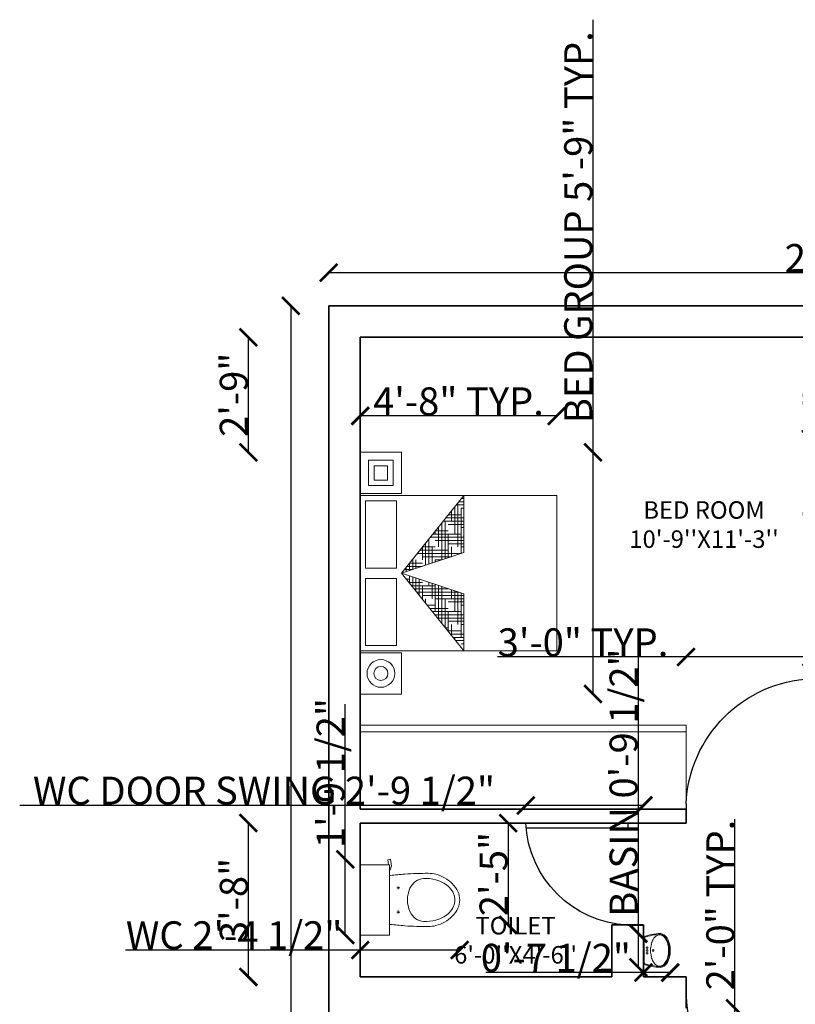
# Model space of a CAD drawing. Units: inches. Extents: x 2435 to 2891, y 1790 to 2334.
# Tile 2 of 3: x 2435 to 2657, y 2052 to 2334. Entities that reach past the tile are written whole.
import ezdxf

# ---------------------------------------------------------------- set-up
doc = ezdxf.new("R2010")
doc.units = ezdxf.units.IN
for name, color, linetype, lineweight in [('A-ANNO-DIMS', 2, 'Continuous', 13), ('A-AREA-IDEN', 7, 'Continuous', 18), ('A-FLOR-FIXT', 9, 'Continuous', 18), ('A-FURN', 8, 'Continuous', 18), ('DOOR', 30, 'Continuous', 25), ('SHELF', 140, 'Continuous', 18), ('WALL', 7, 'Continuous', 35)]:
    doc.layers.add(name, color=color, linetype=linetype, lineweight=lineweight)
doc.styles.get("Standard").update_dxf_attribs({"font": 'arial.ttf'})
doc.dimstyles.get("Standard").update_dxf_attribs({"dimtxt": 8, "dimasz": 5, "dimexe": 0.18, "dimexo": 0.0625, "dimgap": 0.09, "dimtad": 1, "dimdec": 1, "dimzin": 0, "dimdsep": 46, "dimlunit": 4, "dimtxsty": 'Standard', "dimblk": 'ARCHTICK', "dimcen": 0.09, "dimse1": 1, "dimse2": 1, "dimadec": 0, "dimazin": 0, "dimtfac": 1, "dimtdec": 1, "dimtofl": 0, "dimtmove": 0, "dimatfit": 3, "dimfxl": 1, "dimtolj": 1, "dimtzin": 0, "dimarcsym": 0})

# ---------------------------------------------------------------- blocks, each defined once
blk = doc.blocks.new('toilet-1')
at = {"color": 0, "linetype": 'ByBlock'}
for p, q in [((-0.23, -0.02), (-0.23, -0.2116)), ((0.23, -0.02), (-0.23, -0.02)), ((0.23, -0.02), (0.23, -0.2116)), ((-0.23, -0.2116), (0.23, -0.2116)), ((0.1917, -0.2144), (0.2206, -0.225)), ((0.2206, -0.225), (0.266, -0.2187)), ((0.2633, -0.1997), (0.23, -0.2044)), ((0.266, -0.2187), (0.2633, -0.1997)), ((-0.0889, -0.2683), (-0.0697, -0.2683)), ((-0.0793, -0.2587), (-0.0793, -0.2778)), ((0.0889, -0.2683), (0.0698, -0.2683)), ((0.0794, -0.2587), (0.0794, -0.2778)), ((0, -0.6382), (0, -0.6382))]:
    blk.add_line(p, q, dxfattribs=at)
for centre, radius, start, end in [((3.5272, -0.6239), 3.7093, 173.69251, 175.15926), ((-3.527, -0.624), 3.7093, 4.84131, 6.31706), ((1.7368, -0.4519), 1.9109, 175.76982, 180.37578), ((-1.7366, -0.4519), 1.9109, 359.62422, 4.23018), ((-0.0408, -0.4398), 0.0996, 145.14967, 175.88096), ((-0.0312, -0.4465), 0.1114, 113.89968, 145.1485), ((0, -0.5169), 0.1884, 66.09393, 113.90607), ((0.0312, -0.4465), 0.1114, 34.8515, 66.10032), ((0.0409, -0.4398), 0.0996, 4.11904, 34.85033), ((0.0981, -0.4497), 0.2389, 175.88621, 195.59308), ((-0.098, -0.4497), 0.2389, 344.40692, 4.11379), ((0.0353, -0.463), 0.2093, 180.37466, 194.33753), ((0.055, -0.458), 0.2297, 194.33532, 209.62204), ((0.0961, -0.4503), 0.2369, 195.59686, 209.37705), ((-0.096, -0.4503), 0.2369, 330.62295, 344.40314), ((-0.0548, -0.458), 0.2297, 330.37879, 345.66551), ((-0.0351, -0.463), 0.2093, 345.6614, 359.62427), ((0.0647, -0.4524), 0.2409, 209.62726, 224.54888), ((0.0232, -0.4913), 0.1532, 209.38715, 226.54376), ((-0.0231, -0.4913), 0.1532, 313.45624, 330.61285), ((-0.0645, -0.4524), 0.2409, 315.45042, 330.37204), ((0.0178, -0.4986), 0.1751, 224.55199, 245.714), ((0.0152, -0.4997), 0.1416, 226.55015, 246.55272), ((0, -0.5347), 0.1034, 246.54933, 270.0042), ((0, -0.5347), 0.1034, 269.9958, 293.45067), ((-0.0151, -0.4997), 0.1416, 293.44728, 313.44985), ((-0.0176, -0.4986), 0.1751, 294.28649, 315.4485), ((0.0004, -0.538), 0.132, 245.58449, 269.87817), ((-0.0002, -0.538), 0.132, 270.12162, 294.4153)]:
    blk.add_arc(centre, radius, start, end, dxfattribs=at)
blk = doc.blocks.new('wash-3')
at = {"color": 0, "linetype": 'ByBlock'}
blk.add_line((0.23, -0.015), (-0.23, -0.015), dxfattribs=at)
for centre in [(-0.05, -0.066), (0, -0.066), (0, -0.172), (0.05, -0.066)]:
    blk.add_circle(centre, 0.0148, dxfattribs=at)
for centre, radius, start, end in [((0.69, -0.34), 0.991, 159.941, 177.839), ((0.69, -0.34), 0.976, 160.5399, 177.7326), ((-0.096, -0.349), 0.203, 119.8322, 144.1588), ((-0.038, -0.45), 0.319, 103.3619, 119.8322), ((0, -0.61), 0.483, 90, 103.3619), ((0, -0.61), 0.483, 76.6381, 90), ((0.038, -0.45), 0.319, 60.1678, 76.6381), ((0.096, -0.349), 0.203, 35.8412, 60.1678), ((-0.69, -0.34), 0.976, 2.2674, 19.4601), ((-0.69, -0.34), 0.991, 2.161, 20.059), ((-0.12, -0.265), 0.184, 191.7424, 233.4191), ((-0.12, -0.265), 0.169, 192.3358, 233.361), ((-0.183, -0.286), 0.095, 144.1588, 180), ((-0.183, -0.286), 0.095, 180, 215.8412), ((-0.096, -0.223), 0.203, 215.8412, 240.1678), ((0.096, -0.223), 0.203, 299.8322, 324.1588), ((0.12, -0.265), 0.169, 306.639, 347.6642), ((0.12, -0.265), 0.184, 306.5809, 348.2576), ((0.183, -0.286), 0.095, 0, 35.8412), ((0.183, -0.286), 0.095, 324.1588, 0), ((-0.096, -0.223), 0.232, 234.7719, 240.1678), ((-0.096, -0.223), 0.217, 234.8176, 240.1678), ((-0.038, -0.122), 0.348, 240.1678, 256.6381), ((-0.038, -0.122), 0.333, 240.1678, 256.6381), ((-0.038, -0.122), 0.319, 240.1678, 256.6381), ((0, 0.038), 0.513, 256.6381, 270), ((0, 0.038), 0.498, 256.6381, 270), ((0, 0.038), 0.483, 256.6381, 270), ((0, 0.038), 0.483, 270, 283.3619), ((0, 0.038), 0.498, 270, 283.3619), ((0, 0.038), 0.513, 270, 283.3619), ((0.038, -0.122), 0.319, 283.3619, 299.8322), ((0.038, -0.122), 0.333, 283.3619, 299.8322), ((0.038, -0.122), 0.348, 283.3619, 299.8322), ((0.096, -0.223), 0.217, 299.8322, 305.1824), ((0.096, -0.223), 0.232, 299.8322, 305.2281)]:
    blk.add_arc(centre, radius, start, end, dxfattribs=at)
blk = doc.blocks.new('AP0B05')
for p, q in [((35, 100), (35, 880)), ((75, 100), (75, 878.9)), ((35, 100), (35, -20)), ((815, 100), (815, -20))]:
    blk.add_line(p, q)
blk.add_lwpolyline([(35, 100), (75, 100)])
blk.add_arc((-2.4, 62.6), 818.3, 2.62122, 87.37878)
blk = doc.blocks.new('*X3')
at = {"color": 0}
for p, q in [((20.1875, 14.75), (20.1875, 14.7669)), ((20.199, 14.7812), (20.2772, 14.7812)), ((20.25, 14.8125), (20.2772, 14.8125)), ((20.1236, 14.6875), (20.25, 14.6875)), ((20.125, 14.5), (20.125, 14.6893)), ((20.1487, 14.7188), (20.2772, 14.7188)), ((20.1562, 14.625), (20.1562, 14.7281)), ((20.1739, 14.75), (20.2772, 14.75)), ((20.25, 14.3194), (20.25, 14.75)), ((20.0625, 14.2573), (20.0625, 14.6116)), ((20.0938, 14.375), (20.0938, 14.6504)), ((20.0984, 14.6562), (20.125, 14.6562)), ((20.125, 14.5938), (20.2772, 14.5938)), ((20.2188, 14.3091), (20.2188, 14.625)), ((20.25, 14.625), (20.2772, 14.625)), ((19.9727, 14.5), (20.25, 14.5)), ((19.9979, 14.5312), (20.2772, 14.5312)), ((20, 14.2366), (20, 14.5)), ((20.023, 14.5625), (20.2772, 14.5625)), ((20.0312, 14.2469), (20.0312, 14.5727)), ((20.1875, 14.2987), (20.1875, 14.5)), ((19.9062, 14.375), (19.9062, 14.4174)), ((19.9225, 14.4375), (20, 14.4375)), ((19.9476, 14.4688), (20.125, 14.4688)), ((20.125, 14.4062), (20.2772, 14.4062)), ((20.25, 14.4375), (20.2772, 14.4375)), ((19.8125, 14.1744), (19.8125, 14.3008)), ((19.8219, 14.3125), (20.2291, 14.3125)), ((19.8438, 14.1848), (19.8438, 14.3397)), ((19.875, 14.25), (19.875, 14.3785)), ((19.875, 14.3438), (20.2772, 14.3438)), ((19.9688, 14.2262), (19.9688, 14.375)), ((20, 14.375), (20.2772, 14.375)), ((20.1562, 14.2884), (20.1562, 14.375)), ((19.7465, 14.2188), (19.875, 14.2188)), ((19.75, 14.1537), (19.75, 14.2231)), ((19.7716, 14.25), (20, 14.25)), ((19.7812, 14.1641), (19.7812, 14.262)), ((19.7967, 14.2812), (20.125, 14.2812)), ((19.9375, 14.2159), (19.9375, 14.25)), ((19.7188, 14.0726), (19.7188, 14.1136)), ((19.7213, 14.1875), (19.75, 14.1875)), ((19.75, 14.0338), (19.75, 14.1032)), ((19.7018, 14.0938), (19.7786, 14.0938)), ((19.7269, 14.0625), (19.8728, 14.0625)), ((19.752, 14.0312), (19.875, 14.0312)), ((19.7812, 13.9949), (19.7812, 14.0929)), ((19.8125, 14), (19.8125, 14.0825)), ((19.9062, 13.8396), (19.9062, 14.0514)), ((19.9375, 13.8007), (19.9375, 14.0411)), ((19.9688, 13.875), (19.9688, 14.0307)), ((20, 14), (20, 14.0204)), ((19.8275, 13.9375), (20.25, 13.9375)), ((19.875, 13.8784), (19.875, 14)), ((19.875, 13.9688), (20.1557, 13.9688)), ((20, 14), (20.0614, 14)), ((20.0625, 13.6454), (20.0625, 13.9996)), ((20.0938, 13.625), (20.0938, 13.9893)), ((20.125, 13.75), (20.125, 13.9789)), ((20.1562, 13.875), (20.1562, 13.9686)), ((20.25, 13.5), (20.25, 13.9375)), ((19.8526, 13.9062), (20.125, 13.9062)), ((19.8777, 13.875), (20, 13.875)), ((20, 13.8125), (20.2772, 13.8125)), ((20.0312, 13.6842), (20.0312, 13.875)), ((20.125, 13.8438), (20.2772, 13.8438)), ((20.2188, 13.4511), (20.2188, 13.875)), ((20.25, 13.875), (20.2772, 13.875)), ((19.9532, 13.7812), (20.2772, 13.7812)), ((19.9783, 13.75), (20.25, 13.75)), ((20, 13.723), (20, 13.75)), ((20.0035, 13.7188), (20.125, 13.7188)), ((20.1875, 13.49), (20.1875, 13.75)), ((20.0789, 13.625), (20.2772, 13.625)), ((20.125, 13.6562), (20.2772, 13.6562)), ((20.1562, 13.5288), (20.1562, 13.625)), ((20.25, 13.6875), (20.2772, 13.6875)), ((20.104, 13.5938), (20.2772, 13.5938)), ((20.1292, 13.5625), (20.25, 13.5625)), ((20.2046, 13.4688), (20.2772, 13.4688)), ((20.2297, 13.4375), (20.2772, 13.4375)), ((20.25, 13.5), (20.2772, 13.5)), ((20.2549, 13.4062), (20.2772, 13.4062))]:
    blk.add_line(p, q, dxfattribs=at)
blk = doc.blocks.new('MAT-P13')
for p, q in [((-1.17, 0), (-1.17, -0.4)), ((-1.17, 0), (-0.77, 0)), ((-0.77, 0), (-0.77, -0.4)), ((-0.75, 0), (0.75, 0)), ((-0.75, 0), (-0.75, -1.9)), ((0.75, 0), (0.75, -1.9)), ((0.77, 0), (1.17, 0)), ((0.77, 0), (0.77, -0.4)), ((1.17, 0), (1.17, -0.4)), ((-0.7, -0.05), (-0.7, -0.35)), ((-0.7, -0.05), (-0.05, -0.05)), ((-0.05, -0.35), (-0.05, -0.05)), ((0.05, -0.05), (0.7, -0.05)), ((0.05, -0.35), (0.05, -0.05)), ((0.7, -0.05), (0.7, -0.35)), ((-0.7, -0.35), (-0.05, -0.35)), ((0.05, -0.35), (0.7, -0.35)), ((-1.17, -0.4), (-0.77, -0.4)), ((-0.75, -1.0034), (0, -0.4)), ((0, -0.4), (-0.75, -1.0034)), ((0, -0.4), (-0.2, -1.0034)), ((0, -0.4), (0.2, -1.0034)), ((0, -0.4), (0.75, -1.0034)), ((0.77, -0.4), (1.17, -0.4)), ((-0.75, -1.0034), (-0.2, -1.0034)), ((0.2, -1.0034), (0.75, -1.0034)), ((0.75, -1.9), (-0.75, -1.9))]:
    blk.add_line(p, q)
for points in [[(0.8468, -0.0814), (1.0932, -0.0814), (1.0932, -0.3186), (0.8468, -0.3186)], [(0.9015, -0.1361), (1.0385, -0.1361), (1.0385, -0.2639), (0.9015, -0.2639)]]:
    blk.add_lwpolyline(points, close=True)
for radius in [0.1342, 0.0686]:
    blk.add_circle((-0.97, -0.2), radius)
at = {"xscale": -1, "rotation": 90}
blk.add_blockref('*X3', (14.1285, 19.2738), dxfattribs=at)
blk = doc.blocks.new('_ArchTick')
at = {"color": 0, "linetype": 'ByBlock', "const_width": 0.15}
blk.add_lwpolyline([(-0.5, -0.5), (0.5, 0.5)], dxfattribs=at)
blk = doc.blocks.new('*D10')
at = {"layer": 'A-ANNO-DIMS', "color": 0, "lineweight": -2, "transparency": 16777216}
blk.add_line((2523.44, 2261.69), (2799.44, 2261.69), dxfattribs=at)
at = {"layer": 'Defpoints', "color": 0, "transparency": 16777216}
for p in [(2799.44, 2261.69), (2523.44, 2252.2), (2799.44, 2252.2)]:
    blk.add_point(p, dxfattribs=at)
at = {"layer": 'A-ANNO-DIMS', "color": 0, "lineweight": -2, "transparency": 16777216, "xscale": 5, "yscale": 5, "zscale": 5, "rotation": 180}
blk.add_blockref('_ArchTick', (2523.44, 2261.69), dxfattribs=at)
at = {"layer": 'A-ANNO-DIMS', "color": 0, "lineweight": -2, "transparency": 16777216, "xscale": 5, "yscale": 5, "zscale": 5}
blk.add_blockref('_ArchTick', (2799.44, 2261.69), dxfattribs=at)
at = {"layer": 'A-ANNO-DIMS', "color": 0, "transparency": 16777216, "insert": (2661.44, 2265.87), "char_height": 8, "attachment_point": 5}
blk.add_mtext("\\A1;23'", dxfattribs=at)
blk = doc.blocks.new('*D11')
at = {"layer": 'A-ANNO-DIMS', "color": 0, "lineweight": -2, "transparency": 16777216}
blk.add_line((2512.57, 2252.2), (2512.57, 1820.2), dxfattribs=at)
at = {"layer": 'Defpoints', "color": 0, "transparency": 16777216}
for p in [(2523.44, 2252.2), (2512.57, 1820.2), (2523.44, 1820.2)]:
    blk.add_point(p, dxfattribs=at)
at = {"layer": 'A-ANNO-DIMS', "color": 0, "lineweight": -2, "transparency": 16777216, "xscale": 5, "yscale": 5, "zscale": 5}
for p, rotation in [((2512.57, 2252.2), 90), ((2512.57, 1820.2), 270)]:
    blk.add_blockref('_ArchTick', p, dxfattribs=dict(at, rotation=rotation))
at = {"layer": 'A-ANNO-DIMS', "color": 0, "transparency": 16777216, "insert": (2508.39, 2036.2), "char_height": 8, "attachment_point": 5, "rotation": 90}
blk.add_mtext("\\A1;36'", dxfattribs=at)
blk = doc.blocks.new('SHELF-BEDROOM')
for p, q in [((93.19, 0), (93.19, 24)), ((0, 1.9), (93.19, 1.9)), ((0, 0), (93.19, 0))]:
    blk.add_line(p, q)
blk = doc.blocks.new('*D15')
at = {"layer": 'A-ANNO-DIMS', "color": 0, "lineweight": -2, "transparency": 16777216}
for p, q in [((2667.64, 2145.53), (2667.64, 2254.35)), ((2667.64, 2104.2), (2667.64, 2145.53))]:
    blk.add_line(p, q, dxfattribs=at)
at = {"layer": 'Defpoints', "color": 0, "transparency": 16777216}
for p in [(2661.44, 2145.53), (2667.64, 2145.53), (2661.44, 2104.2)]:
    blk.add_point(p, dxfattribs=at)
at = {"layer": 'A-ANNO-DIMS', "color": 0, "lineweight": -2, "transparency": 16777216, "xscale": 5, "yscale": 5, "zscale": 5}
for p, rotation in [((2667.64, 2145.53), 90), ((2667.64, 2104.2), 270)]:
    blk.add_blockref('_ArchTick', p, dxfattribs=dict(at, rotation=rotation))
at = {"layer": 'A-ANNO-DIMS', "color": 0, "transparency": 16777216, "insert": (2663.41, 2202.44), "char_height": 8, "attachment_point": 5, "rotation": 90}
blk.add_mtext('\\A1;DOOR 3\'-5 1/2" TYP.', dxfattribs=at)
blk = doc.blocks.new('*D16')
at = {"layer": 'A-ANNO-DIMS', "color": 0, "lineweight": -2, "transparency": 16777216}
for p, q in [((2625.63, 2151.73), (2571.69, 2151.73)), ((2661.44, 2151.73), (2625.63, 2151.73))]:
    blk.add_line(p, q, dxfattribs=at)
at = {"layer": 'Defpoints', "color": 0, "transparency": 16777216}
for p in [(2625.63, 2151.73), (2625.63, 2145.53), (2661.44, 2145.53)]:
    blk.add_point(p, dxfattribs=at)
at = {"layer": 'A-ANNO-DIMS', "color": 0, "lineweight": -2, "transparency": 16777216, "xscale": 5, "yscale": 5, "zscale": 5, "rotation": 180}
blk.add_blockref('_ArchTick', (2625.63, 2151.73), dxfattribs=at)
at = {"layer": 'A-ANNO-DIMS', "color": 0, "lineweight": -2, "transparency": 16777216, "xscale": 5, "yscale": 5, "zscale": 5}
blk.add_blockref('_ArchTick', (2661.44, 2151.73), dxfattribs=at)
at = {"layer": 'A-ANNO-DIMS', "color": 0, "transparency": 16777216, "insert": (2596.16, 2155.91), "char_height": 8, "attachment_point": 5}
blk.add_mtext('\\A1;3\'-0" TYP.', dxfattribs=at)
blk = doc.blocks.new('*D19')
at = {"layer": 'A-ANNO-DIMS', "color": 0, "lineweight": -2, "transparency": 16777216}
for p, q in [((2579.79, 2109.25), (2435.04, 2109.25)), ((2613.44, 2109.25), (2579.79, 2109.25))]:
    blk.add_line(p, q, dxfattribs=at)
at = {"layer": 'Defpoints', "color": 0, "transparency": 16777216}
for p in [(2579.79, 2109.25), (2579.79, 2104.2), (2613.44, 2104.2)]:
    blk.add_point(p, dxfattribs=at)
at = {"layer": 'A-ANNO-DIMS', "color": 0, "lineweight": -2, "transparency": 16777216, "xscale": 5, "yscale": 5, "zscale": 5, "rotation": 180.0000000000007}
blk.add_blockref('_ArchTick', (2579.79, 2109.25), dxfattribs=at)
at = {"layer": 'A-ANNO-DIMS', "color": 0, "lineweight": -2, "transparency": 16777216, "xscale": 5, "yscale": 5, "zscale": 5}
blk.add_blockref('_ArchTick', (2613.44, 2109.25), dxfattribs=at)
at = {"layer": 'A-ANNO-DIMS', "color": 0, "transparency": 16777216, "insert": (2504.92, 2113.48), "char_height": 8, "attachment_point": 5}
blk.add_mtext('\\A1;WC DOOR SWING 2\'-9 1/2"', dxfattribs=at)
blk = doc.blocks.new('*D20')
at = {"layer": 'A-ANNO-DIMS', "color": 0, "lineweight": -2, "transparency": 16777216}
blk.add_line((2574.75, 2104.2), (2574.75, 2075.04), dxfattribs=at)
at = {"layer": 'Defpoints', "color": 0, "transparency": 16777216}
for p in [(2579.79, 2104.2), (2574.75, 2075.04), (2579.79, 2075.04)]:
    blk.add_point(p, dxfattribs=at)
at = {"layer": 'A-ANNO-DIMS', "color": 0, "lineweight": -2, "transparency": 16777216, "xscale": 5, "yscale": 5, "zscale": 5}
for p, rotation in [((2574.75, 2104.2), 90), ((2574.75, 2075.04), 270)]:
    blk.add_blockref('_ArchTick', p, dxfattribs=dict(at, rotation=rotation))
at = {"layer": 'A-ANNO-DIMS', "color": 0, "transparency": 16777216, "insert": (2570.57, 2089.62), "char_height": 8, "attachment_point": 5, "rotation": 90}
blk.add_mtext('\\A1;2\'-5"', dxfattribs=at)
blk = doc.blocks.new('*D23')
at = {"layer": 'A-ANNO-DIMS', "color": 0, "lineweight": -2, "transparency": 16777216}
for p, q in [((2599.02, 2210.31), (2599.02, 2334.07)), ((2599.02, 2141.1), (2599.02, 2210.31))]:
    blk.add_line(p, q, dxfattribs=at)
at = {"layer": 'Defpoints', "color": 0, "transparency": 16777216}
for p in [(2588.64, 2210.31), (2599.02, 2210.31), (2588.64, 2141.1)]:
    blk.add_point(p, dxfattribs=at)
at = {"layer": 'A-ANNO-DIMS', "color": 0, "lineweight": -2, "transparency": 16777216, "xscale": 5, "yscale": 5, "zscale": 5}
for p, rotation in [((2599.02, 2210.31), 90), ((2599.02, 2141.1), 270)]:
    blk.add_blockref('_ArchTick', p, dxfattribs=dict(at, rotation=rotation))
at = {"layer": 'A-ANNO-DIMS', "color": 0, "transparency": 16777216, "insert": (2594.79, 2274.69), "char_height": 8, "attachment_point": 5, "rotation": 90}
blk.add_mtext('\\A1;BED GROUP 5\'-9" TYP.', dxfattribs=at)
blk = doc.blocks.new('*D24')
at = {"layer": 'A-ANNO-DIMS', "color": 0, "lineweight": -2, "transparency": 16777216}
blk.add_line((2588.64, 2220.69), (2532.44, 2220.69), dxfattribs=at)
at = {"layer": 'Defpoints', "color": 0, "transparency": 16777216}
for p in [(2532.44, 2220.69), (2532.44, 2210.31), (2588.64, 2210.31)]:
    blk.add_point(p, dxfattribs=at)
at = {"layer": 'A-ANNO-DIMS', "color": 0, "lineweight": -2, "transparency": 16777216, "xscale": 5, "yscale": 5, "zscale": 5, "rotation": 180}
blk.add_blockref('_ArchTick', (2532.44, 2220.69), dxfattribs=at)
at = {"layer": 'A-ANNO-DIMS', "color": 0, "lineweight": -2, "transparency": 16777216, "xscale": 5, "yscale": 5, "zscale": 5}
blk.add_blockref('_ArchTick', (2588.64, 2220.69), dxfattribs=at)
at = {"layer": 'A-ANNO-DIMS', "color": 0, "transparency": 16777216, "insert": (2560.54, 2224.87), "char_height": 8, "attachment_point": 5}
blk.add_mtext('\\A1;4\'-8" TYP.', dxfattribs=at)
blk = doc.blocks.new('*D28')
at = {"layer": 'A-ANNO-DIMS', "color": 0, "lineweight": -2, "transparency": 16777216}
for p, q in [((2639.61, 2051.2), (2639.61, 2105.28)), ((2639.61, 2027.2), (2639.61, 2051.2))]:
    blk.add_line(p, q, dxfattribs=at)
at = {"layer": 'Defpoints', "color": 0, "transparency": 16777216}
for p in [(2625.63, 2051.2), (2639.61, 2051.2), (2625.63, 2027.2)]:
    blk.add_point(p, dxfattribs=at)
at = {"layer": 'A-ANNO-DIMS', "color": 0, "lineweight": -2, "transparency": 16777216, "xscale": 5, "yscale": 5, "zscale": 5}
for p, rotation in [((2639.61, 2051.2), 90), ((2639.61, 2027.2), 270)]:
    blk.add_blockref('_ArchTick', p, dxfattribs=dict(at, rotation=rotation))
at = {"layer": 'A-ANNO-DIMS', "color": 0, "transparency": 16777216, "insert": (2635.43, 2080.74), "char_height": 8, "attachment_point": 5, "rotation": 90}
blk.add_mtext('\\A1;2\'-0" TYP.', dxfattribs=at)
blk = doc.blocks.new('*D35')
at = {"layer": 'A-ANNO-DIMS', "color": 0, "lineweight": -2, "transparency": 16777216}
for p, q in [((2532.44, 2067.87), (2465.31, 2067.87)), ((2560.89, 2067.87), (2532.44, 2067.87))]:
    blk.add_line(p, q, dxfattribs=at)
at = {"layer": 'Defpoints', "color": 0, "transparency": 16777216}
for p in [(2532.44, 2072.14), (2560.89, 2072.14), (2532.44, 2067.87)]:
    blk.add_point(p, dxfattribs=at)
at = {"layer": 'A-ANNO-DIMS', "color": 0, "lineweight": -2, "transparency": 16777216, "xscale": 5, "yscale": 5, "zscale": 5, "rotation": 180}
blk.add_blockref('_ArchTick', (2532.44, 2067.87), dxfattribs=at)
at = {"layer": 'A-ANNO-DIMS', "color": 0, "lineweight": -2, "transparency": 16777216, "xscale": 5, "yscale": 5, "zscale": 5}
blk.add_blockref('_ArchTick', (2560.89, 2067.87), dxfattribs=at)
at = {"layer": 'A-ANNO-DIMS', "color": 0, "transparency": 16777216, "insert": (2496.38, 2072.1), "char_height": 8, "attachment_point": 5}
blk.add_mtext('\\A1;WC 2\'-4 1/2"', dxfattribs=at)
blk = doc.blocks.new('*D36')
at = {"layer": 'A-ANNO-DIMS', "color": 0, "lineweight": -2, "transparency": 16777216}
for p, q in [((2528.18, 2093.85), (2528.18, 2138.18)), ((2528.18, 2072.14), (2528.18, 2093.85))]:
    blk.add_line(p, q, dxfattribs=at)
at = {"layer": 'Defpoints', "color": 0, "transparency": 16777216}
for p in [(2528.18, 2093.85), (2532.44, 2093.85), (2532.44, 2072.14)]:
    blk.add_point(p, dxfattribs=at)
at = {"layer": 'A-ANNO-DIMS', "color": 0, "lineweight": -2, "transparency": 16777216, "xscale": 5, "yscale": 5, "zscale": 5}
for p, rotation in [((2528.18, 2093.85), 90), ((2528.18, 2072.14), 270)]:
    blk.add_blockref('_ArchTick', p, dxfattribs=dict(at, rotation=rotation))
at = {"layer": 'A-ANNO-DIMS', "color": 0, "transparency": 16777216, "insert": (2523.95, 2118.51), "char_height": 8, "attachment_point": 5, "rotation": 90}
blk.add_mtext('\\A1;1\'-9 1/2"', dxfattribs=at)
blk = doc.blocks.new('*D37')
at = {"layer": 'A-ANNO-DIMS', "color": 0, "lineweight": -2, "transparency": 16777216}
for p, q in [((2611.99, 2072.6), (2611.99, 2153.97)), ((2611.99, 2062.89), (2611.99, 2072.6))]:
    blk.add_line(p, q, dxfattribs=at)
at = {"layer": 'Defpoints', "color": 0, "transparency": 16777216}
for p in [(2611.99, 2072.6), (2613.44, 2072.6), (2613.44, 2062.89)]:
    blk.add_point(p, dxfattribs=at)
at = {"layer": 'A-ANNO-DIMS', "color": 0, "lineweight": -2, "transparency": 16777216, "xscale": 5, "yscale": 5, "zscale": 5}
for p, rotation in [((2611.99, 2072.6), 90), ((2611.99, 2062.89), 270)]:
    blk.add_blockref('_ArchTick', p, dxfattribs=dict(at, rotation=rotation))
at = {"layer": 'A-ANNO-DIMS', "color": 0, "transparency": 16777216, "insert": (2607.76, 2115.79), "char_height": 8, "attachment_point": 5, "rotation": 90}
blk.add_mtext('\\A1;BASIN 0\'-9 1/2"', dxfattribs=at)
blk = doc.blocks.new('*D38')
at = {"layer": 'A-ANNO-DIMS', "color": 0, "lineweight": -2, "transparency": 16777216}
for p, q in [((2613.44, 2061.44), (2568.36, 2061.44)), ((2621.13, 2061.44), (2613.44, 2061.44))]:
    blk.add_line(p, q, dxfattribs=at)
at = {"layer": 'Defpoints', "color": 0, "transparency": 16777216}
for p in [(2613.44, 2062.89), (2621.13, 2062.89), (2613.44, 2061.44)]:
    blk.add_point(p, dxfattribs=at)
at = {"layer": 'A-ANNO-DIMS', "color": 0, "lineweight": -2, "transparency": 16777216, "xscale": 5, "yscale": 5, "zscale": 5, "rotation": 180}
blk.add_blockref('_ArchTick', (2613.44, 2061.44), dxfattribs=at)
at = {"layer": 'A-ANNO-DIMS', "color": 0, "lineweight": -2, "transparency": 16777216, "xscale": 5, "yscale": 5, "zscale": 5}
blk.add_blockref('_ArchTick', (2621.13, 2061.44), dxfattribs=at)
at = {"layer": 'A-ANNO-DIMS', "color": 0, "transparency": 16777216, "insert": (2588.4, 2065.66), "char_height": 8, "attachment_point": 5}
blk.add_mtext('\\A1;0\'-7 1/2"', dxfattribs=at)
blk = doc.blocks.new('*D45')
at = {"layer": 'A-ANNO-DIMS', "color": 0, "lineweight": -2, "transparency": 16777216}
blk.add_line((2500.44, 2060.2), (2500.44, 2104.2), dxfattribs=at)
at = {"layer": 'Defpoints', "color": 0, "transparency": 16777216}
for p in [(2500.44, 2104.2), (2532.44, 2104.2), (2532.44, 2060.2)]:
    blk.add_point(p, dxfattribs=at)
at = {"layer": 'A-ANNO-DIMS', "color": 0, "lineweight": -2, "transparency": 16777216, "xscale": 5, "yscale": 5, "zscale": 5}
for p, rotation in [((2500.44, 2104.2), 90), ((2500.44, 2060.2), 270)]:
    blk.add_blockref('_ArchTick', p, dxfattribs=dict(at, rotation=rotation))
at = {"layer": 'A-ANNO-DIMS', "color": 0, "transparency": 16777216, "insert": (2496.27, 2082.2), "char_height": 8, "attachment_point": 5, "rotation": 90}
blk.add_mtext('\\A1;3\'-8"', dxfattribs=at)
blk = doc.blocks.new('*D46')
at = {"layer": 'A-ANNO-DIMS', "color": 0, "lineweight": -2, "transparency": 16777216}
for p, q in [((2822.44, 2075.04), (2822.44, 2100.73)), ((2822.44, 2060.2), (2822.44, 2075.04))]:
    blk.add_line(p, q, dxfattribs=at)
at = {"layer": 'Defpoints', "color": 0, "transparency": 16777216}
for p in [(2604.44, 2075.04), (2822.44, 2075.04), (2604.44, 2060.2)]:
    blk.add_point(p, dxfattribs=at)
at = {"layer": 'A-ANNO-DIMS', "color": 0, "lineweight": -2, "transparency": 16777216, "xscale": 5, "yscale": 5, "zscale": 5}
for p, rotation in [((2822.44, 2075.04), 90), ((2822.44, 2060.2), 270)]:
    blk.add_blockref('_ArchTick', p, dxfattribs=dict(at, rotation=rotation))
at = {"layer": 'A-ANNO-DIMS', "color": 0, "transparency": 16777216, "insert": (2818.27, 2090.39), "char_height": 8, "attachment_point": 5, "rotation": 90}
blk.add_mtext('\\A1;1\'-3"', dxfattribs=at)
blk = doc.blocks.new('*D58')
at = {"layer": 'A-ANNO-DIMS', "color": 0, "lineweight": -2, "transparency": 16777216}
blk.add_line((2500.44, 2210.31), (2500.44, 2243.2), dxfattribs=at)
at = {"layer": 'Defpoints', "color": 0, "transparency": 16777216}
for p in [(2500.44, 2243.2), (2532.44, 2243.2), (2532.44, 2210.31)]:
    blk.add_point(p, dxfattribs=at)
at = {"layer": 'A-ANNO-DIMS', "color": 0, "lineweight": -2, "transparency": 16777216, "xscale": 5, "yscale": 5, "zscale": 5}
for p, rotation in [((2500.44, 2243.2), 90), ((2500.44, 2210.31), 270)]:
    blk.add_blockref('_ArchTick', p, dxfattribs=dict(at, rotation=rotation))
at = {"layer": 'A-ANNO-DIMS', "color": 0, "transparency": 16777216, "insert": (2496.27, 2226.76), "char_height": 8, "attachment_point": 5, "rotation": 90}
blk.add_mtext('\\A1;2\'-9"', dxfattribs=at)

msp = doc.modelspace()

# ---------------------------------------------------------------- linework, layer by layer
at = {"layer": 'WALL'}
for p, q in [((2523.44, 2252.2), (2799.44, 2252.2)), ((2523.44, 2252.2), (2523.44, 1820.2)), ((2532.44, 2243.2), (2670.44, 2243.2)), ((2532.44, 2243.2), (2532.44, 2108.2)), ((2532.44, 2108.2), (2625.63, 2108.2)), ((2625.63, 2104.2), (2625.63, 2108.2)), ((2532.44, 2104.2), (2625.63, 2104.2)), ((2532.44, 2104.2), (2532.44, 2060.2)), ((2604.44, 2075.04), (2613.44, 2075.04)), ((2604.44, 2075.04), (2604.44, 2060.2)), ((2613.44, 2075.04), (2613.44, 2060.2)), ((2532.44, 2060.2), (2604.44, 2060.2)), ((2613.44, 2060.2), (2625.63, 2060.2)), ((2625.63, 2060.2), (2625.63, 2051.2))]:
    msp.add_line(p, q, dxfattribs=at)

# ---------------------------------------------------------------- block references
at = {"layer": 'A-FLOR-FIXT', "rotation": 90}
for name, p, xscale, yscale, zscale in [('toilet-1', (2531.57, 2082.2), 43.76607636236935, 43.76607636236935, 43.76607636236935), ('wash-3', (2613.44, 2067.75), 16.17213832521055, 16.17213832521055, 16.17213832521055)]:
    msp.add_blockref(name, p, dxfattribs=dict(at, xscale=xscale, yscale=yscale, zscale=zscale))
at = {"layer": 'A-FURN', "xscale": 29.57686120969658, "yscale": 29.57686120969658, "zscale": 29.57686120969658, "rotation": 90}
msp.add_blockref('MAT-P13', (2532.44, 2175.7), dxfattribs=at)
at = {"layer": 'DOOR', "xscale": -0.0459165349072543, "yscale": 0.0459165349072543, "zscale": 0.0459165349072543}
msp.add_blockref('AP0B05', (2663.05, 2105.12), dxfattribs=at)
at = {"layer": 'DOOR'}
for p, xscale, yscale, zscale, rotation in [((2612.7, 2105.51), -0.0373902694163411, 0.0373902694163411, 0.0373902694163411, 90.00000000000072), ((2663.05, 2059.29), 0.0459165349072538, 0.0459165349072538, 0.0459165349072538, 180)]:
    msp.add_blockref('AP0B05', p, dxfattribs=dict(at, xscale=xscale, yscale=yscale, zscale=zscale, rotation=rotation))
at = {"layer": 'SHELF', "extrusion": (0, 0, -1), "zscale": -1, "rotation": 180}
msp.add_blockref('SHELF-BEDROOM', (-2532.44, 2132.2), dxfattribs=at)

# ---------------------------------------------------------------- texts
at = {"layer": 'A-AREA-IDEN', "char_height": 5, "attachment_point": 1}
for s, insert in [("\\pxqc;BED ROOM\\P10'-9''X11'-3''", (2612.13, 2196.28)), ("\\pxqc;TOILET\\P6'-0''X4'-6''", (2558.23, 2077.34))]:
    msp.add_mtext_dynamic_manual_height_columns(s, width=37.2819, gutter_width=12.5, heights=[0], dxfattribs=dict(at, insert=insert))

# ---------------------------------------------------------------- dimensions: what is measured, and where the dimension line sits
at = {"layer": 'A-ANNO-DIMS'}
for base, p1, p2, angle, text, picture, middle in [((2599.02, 2210.31), (2588.64, 2141.1), (2588.64, 2210.31), 90, 'BED GROUP <> TYP.', '*D23', (2594.79, 2274.69)), ((2667.64, 2145.53), (2661.44, 2104.2), (2661.44, 2145.53), 90, 'DOOR <> TYP.', '*D15', (2663.41, 2202.44)), ((2532.44, 2220.69), (2588.64, 2210.31), (2532.44, 2210.31), 180, '<> TYP.', '*D24', (2560.54, 2224.87)), ((2625.63, 2151.73), (2661.44, 2145.53), (2625.63, 2145.53), 180, '<> TYP.', '*D16', (2596.16, 2155.91)), ((2611.99, 2072.6), (2613.44, 2062.89), (2613.44, 2072.6), 90, 'BASIN <>', '*D37', (2607.76, 2115.79)), ((2579.7937, 2109.2519), (2613.4449, 2104.2042), (2579.7937, 2104.2042), 180, 'WC DOOR SWING <>', '*D19', (2504.9192, 2113.481)), ((2639.61, 2051.2), (2625.63, 2027.2), (2625.63, 2051.2), 90, '<> TYP.', '*D28', (2635.43, 2080.74)), ((2532.4449, 2067.8708), (2560.8929, 2072.138), (2532.4449, 2072.138), 180, 'WC <>', '*D35', (2496.3754, 2072.0972))]:
    dim = msp.add_linear_dim(base=base, p1=p1, p2=p2, angle=angle, text=text, dimstyle='Standard', override={"dimdec": 1, "dimlfac": 1, "dimrnd": 0, "dimzin": 1, "dimdsep": 46, "dimlunit": 4, "dimfrac": 2}, dxfattribs=at)
    dim.commit()
    dim.dimension.update_dxf_attribs({"geometry": picture, "text_midpoint": middle})
dim = msp.add_linear_dim(base=(2799.44, 2261.69), p1=(2523.44, 2252.2), p2=(2799.44, 2252.2), dimstyle='Standard', override={"dimclrd": 0, "dimclre": 0, "dimclrt": 0}, dxfattribs=at)
dim.commit()
dim.dimension.update_dxf_attribs({"geometry": '*D10', "text_midpoint": (2661.44, 2265.87)})
for base, p1, p2, angle, override, picture, middle in [((2512.57, 1820.2), (2523.44, 2252.2), (2523.44, 1820.2), 90, {"dimclrd": 0, "dimclre": 0, "dimclrt": 0}, '*D11', (2508.39, 2036.2)), ((2500.44, 2243.2), (2532.44, 2210.31), (2532.44, 2243.2), 90, {"dimdec": 1, "dimlfac": 1, "dimrnd": 0, "dimzin": 1, "dimdsep": 46, "dimlunit": 4, "dimfrac": 2}, '*D58', (2496.27, 2226.76)), ((2528.18, 2093.85), (2532.44, 2072.14), (2532.44, 2093.85), 90, {"dimdec": 1, "dimlfac": 1, "dimrnd": 0, "dimzin": 1, "dimdsep": 46, "dimlunit": 4, "dimfrac": 2}, '*D36', (2523.95, 2118.51)), ((2500.44, 2104.2), (2532.44, 2060.2), (2532.44, 2104.2), 90, {"dimdec": 1, "dimlfac": 1, "dimrnd": 0, "dimzin": 1, "dimdsep": 46, "dimlunit": 4, "dimfrac": 2}, '*D45', (2496.27, 2082.2)), ((2574.75, 2075.04), (2579.79, 2104.2), (2579.79, 2075.04), 270, {"dimdec": 1, "dimlfac": 1, "dimrnd": 0, "dimzin": 1, "dimdsep": 46, "dimlunit": 4, "dimfrac": 2}, '*D20', (2570.57, 2089.62)), ((2822.44, 2075.04), (2604.44, 2060.2), (2604.44, 2075.04), 90, {"dimdec": 1, "dimlfac": 1, "dimrnd": 0, "dimzin": 1, "dimdsep": 46, "dimlunit": 4, "dimfrac": 2}, '*D46', (2818.27, 2090.39)), ((2613.44, 2061.44), (2621.13, 2062.89), (2613.44, 2062.89), 180, {"dimdec": 1, "dimlfac": 1, "dimrnd": 0, "dimzin": 1, "dimdsep": 46, "dimlunit": 4, "dimfrac": 2}, '*D38', (2588.4, 2065.66))]:
    dim = msp.add_linear_dim(base=base, p1=p1, p2=p2, angle=angle, dimstyle='Standard', override=override, dxfattribs=at)
    dim.commit()
    dim.dimension.update_dxf_attribs({"geometry": picture, "text_midpoint": middle})

doc.saveas('drawing.dxf')
